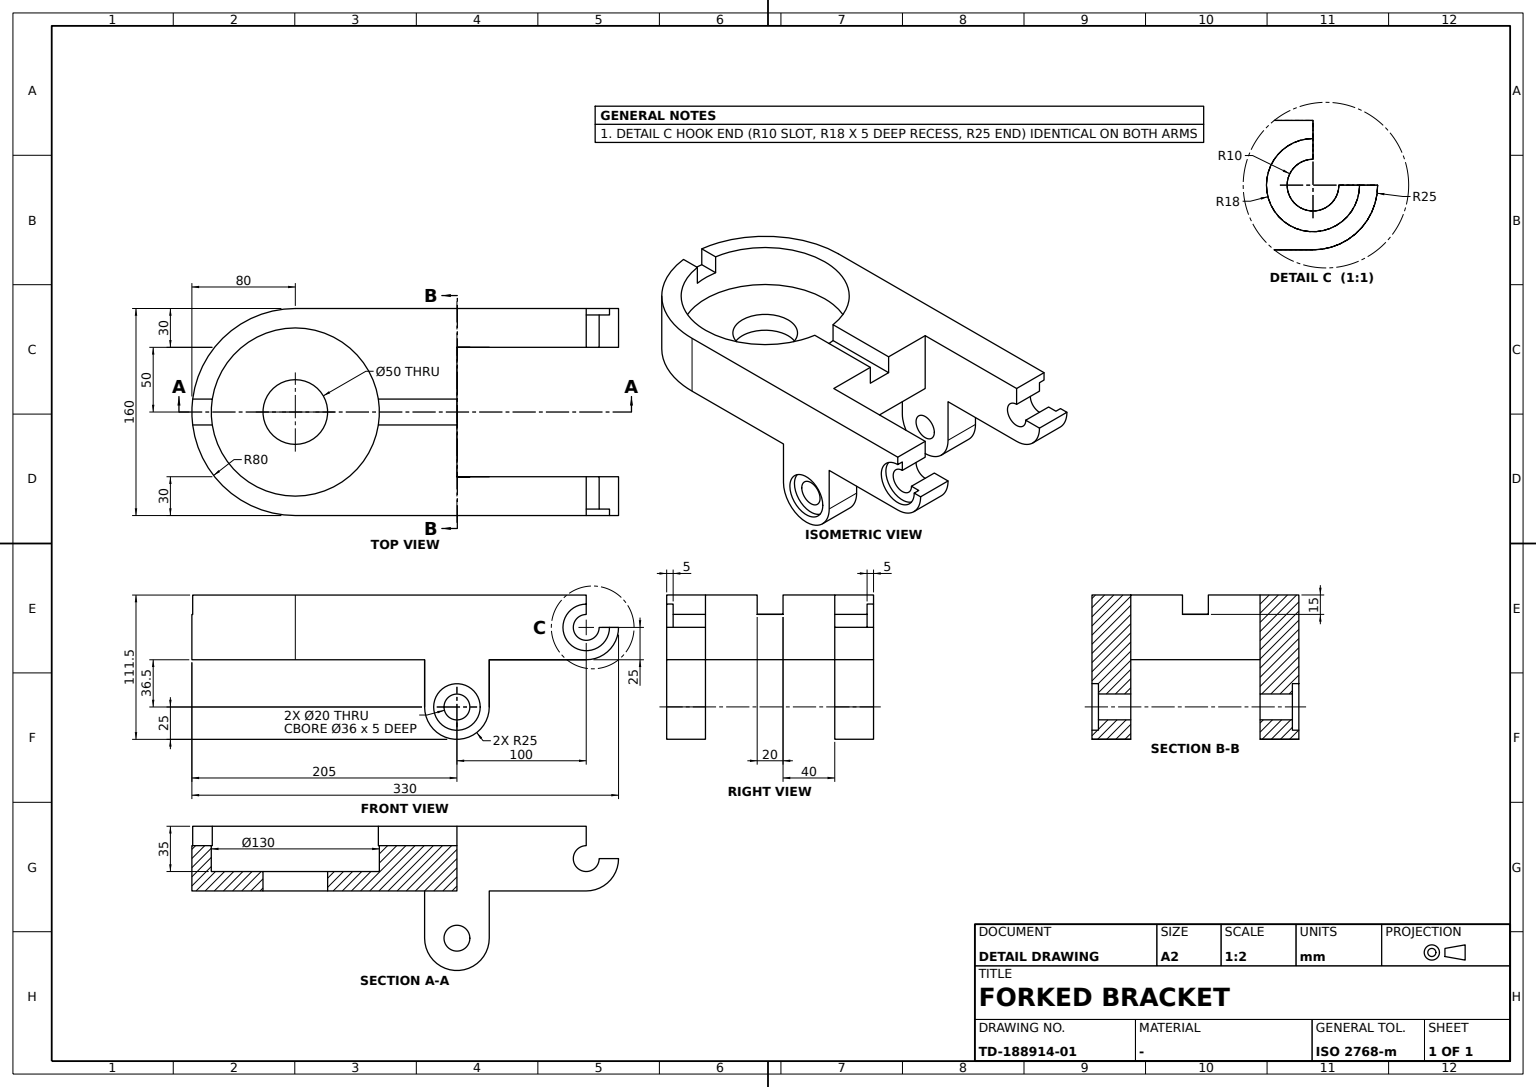
CATIA V5 part; units mm, degrees
sketch "Sketch1" plane through (0, 0, 0) normal (1, 0, 0) x (0, 1, 0)
  line L0 (0, 0) -> (-100, 0)
  line L1 (-100, 0) -> (-100, 50)
  line L2 (0, 0) -> (0, -36.5)
  line L3 (50, -36.5) -> (50, 0)
  point P0 (50, 0)
  line L4 (50, 0) -> (125, 0)
  point P1 (125, 0)
  line L5 (-100, 50) -> (125, 50)
  line L6 (125, 50) -> (125, 0)
  arc A0 (0, -36.5) -> (50, -36.5) centre (25, -36.5) ccw
  dimension "length L0" = 100
  dimension "length L1" = 50
  dimension "length L2" = 36.5
  dimension "distance L3 L2" = 50
  dimension "distance P1 L3" = 75
  dimension "radius A0" = 25
  constraint horizontal L0 x-axis
  constraint horizontal L4 x-axis
  constraint horizontal L5 x-axis
  constraint vertical L1 y-axis
  constraint vertical L2 y-axis
  constraint vertical L3 y-axis
  constraint vertical L6 y-axis
  constraint coincidence P0 x-axis
  constraint tangency A0 L2
extrude "Pad1" add sketch "Sketch1" along normal mid plane 160
sketch "Sketch2" plane through (0, 0, 50) normal (0, 0, 1) x (1, 0, 0)
  arc A0 (-80, -100) -> (80, -100) centre (0, -100.0001) ccw
  point P0 (0, -100.0001)
  line L0 (-80, -100) -> (80, -100)
  dimension "radius A0" = 80
  dimension "length L0" = 160
  dimension "distance L0 x axis" = 100
  constraint horizontal L0 x-axis
  constraint coincidence P0 y-axis
extrude "Pad2" add sketch "Sketch2" against normal blind 50
sketch "Sketch3" plane through (0, 0, 50) normal (0, 0, 1) x (1, 0, 0)
  circle A0 centre (0, -100.0001) radius 65
  arc A1 (-80, -100) -> (80, -100) centre (0, -100.0001) ccw construction
  dimension "radius A0" = 65
  constraint concentricity A0 A1
extrude "Pocket1" cut sketch "Sketch3" against normal blind 35
sketch "Sketch4" plane through (0, 0, 15) normal (0, 0, 1) x (1, 0, 0)
  circle A0 centre (0, -100.0001) radius 25
  point P0 (0, -100.0001)
  circle A1 centre (0, -100.0001) radius 65 construction
  dimension "radius A0" = 25
  constraint coincidence P0 y-axis
  constraint concentricity A0 A1
extrude "Pocket2" cut sketch "Sketch4" against normal blind 35
sketch "Sketch5" plane through (0, 0, 50) normal (0, 0, 1) x (1, 0, 0)
  point P0 (0, -89.1241)
  line L0 (10, 25) -> (10, -203.2481)
  line L1 (10, -203.2481) -> (-10, -203.2481)
  line L2 (-10, -203.2481) -> (-10, 25)
  line L3 (-10, 25) -> (10, 25)
  line L4 (-80, 125) -> (80, 125) construction
  dimension "length L1" = 20
  dimension "distance L3 L4" = 100
  constraint coincidence P0 y-axis
  constraint vertical L0 y-axis
  constraint vertical L2 y-axis
  constraint horizontal L1 x-axis
  constraint horizontal L3 x-axis
  constraint equidistance L0 L2 P0
  constraint equidistance L1 L3 P0
extrude "Pocket3" cut sketch "Sketch5" against normal blind 15
sketch "Sketch6" plane through (0, 0, 50) normal (0, 0, 1) x (1, 0, 0)
  point P0 (0, 76.7365)
  line L0 (50, 128.4731) -> (50, 25)
  line L1 (50, 25) -> (-50, 25)
  line L2 (-50, 25) -> (-50, 128.4731)
  line L3 (-50, 128.4731) -> (50, 128.4731)
  line L4 (80, 125) -> (80, -100) construction
  line L5 (10, 25) -> (-10, 25) construction
  dimension "distance L0 L4" = 30
  constraint coincidence P0 y-axis
  constraint coincidence L1 L5
  constraint vertical L0 y-axis
  constraint vertical L2 y-axis
  constraint horizontal L1 x-axis
  constraint horizontal L3 x-axis
  constraint equidistance L0 L2 P0
  constraint equidistance L1 L3 P0
extrude "Pocket4" cut sketch "Sketch6" against normal through all
sketch "Sketch7" plane through (0, 25, 0) normal (0, 1, 0) x (-1, 0, 0)
  point P0 (0, -36.8491)
  line L0 (50, 0) -> (50, -73.6983)
  line L1 (50, -73.6983) -> (-50, -73.6983)
  line L2 (-50, -73.6983) -> (-50, 0)
  line L3 (-50, 0) -> (50, 0)
  line L4 (80, 0) -> (-80, 0) construction
  line L5 (50, -36.5) -> (50, 0) construction
  constraint coincidence P0 y-axis
  constraint coincidence L3 L4
  constraint coincidence L0 L5
  constraint vertical L0 y-axis
  constraint vertical L2 y-axis
  constraint horizontal L1 x-axis
  constraint horizontal L3 x-axis
  constraint equidistance L0 L2 P0
  constraint equidistance L1 L3 P0
extrude "Pocket5" cut sketch "Sketch7" against normal through all
sketch "Sketch8" plane through (80, 0, 0) normal (1, 0, 0) x (0, 1, 0)
  circle A0 centre (125, 25) radius 25
  point P0 (125, 25)
  line L0 (125, 0) -> (125, 50) construction
  line L1 (125, 50) -> (-100, 50) construction
  line L2 (50, 0) -> (125, 0) construction
  dimension "distance P0 L1" = 25
  constraint coincidence P0 L0
  constraint tangency A0 L2
extrude "Pad3" add sketch "Sketch8" against normal blind 30
mirror "Mirror1" about plane through (0, 0, 0) normal (1, 0, 0) of "Pad3"
sketch "Sketch9" plane through (80, 0, 0) normal (1, 0, 0) x (0, 1, 0)
  circle A0 centre (125, 25) radius 18
  circle A1 centre (125, 25) radius 25 construction
  dimension "radius A0" = 18
  constraint concentricity A1 A0
extrude "Pocket6" cut sketch "Sketch9" against normal blind 5
mirror "Mirror2" about plane through (0, 0, 0) normal (1, 0, 0) of "Pocket6"
sketch "Sketch10" plane through (80, 0, 0) normal (1, 0, 0) x (0, 1, 0)
  line L0 (125, 25) -> (161.9821, 25)
  line L1 (125, 25) -> (125, 71.5934)
  line L2 (125, 71.5934) -> (161.9821, 25)
  constraint horizontal L0 x-axis
  constraint vertical L1 y-axis
extrude "Pocket7" cut sketch "Sketch10" against normal through all
sketch "Sketch11" plane through (75, 0, 0) normal (1, 0, 0) x (0, 1, 0)
  circle A0 centre (125, 25) radius 10
  circle A1 centre (125, 25) radius 18 construction
  dimension "radius A0" = 10
  constraint concentricity A0 A1
extrude "Pocket8" cut sketch "Sketch11" against normal through all
sketch "Sketch12" plane through (80, 0, 0) normal (1, 0, 0) x (0, 1, 0)
  circle A0 centre (25, -36.5) radius 10
  arc A1 (0, -36.5) -> (50, -36.5) centre (25, -36.5) ccw construction
  dimension "radius A0" = 10
  constraint concentricity A0 A1
extrude "Pocket9" cut sketch "Sketch12" against normal through all
sketch "Sketch13" plane through (80, 0, 0) normal (1, 0, 0) x (0, 1, 0)
  circle A0 centre (25, -36.5) radius 18
  circle A1 centre (25, -36.5) radius 10 construction
  dimension "radius A0" = 18
  constraint concentricity A0 A1
extrude "Pocket10" cut sketch "Sketch13" against normal blind 5
mirror "Mirror3" about plane through (0, 0, 0) normal (1, 0, 0) of "Pocket10"
